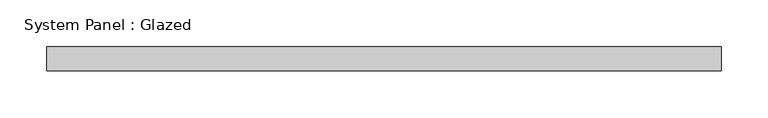
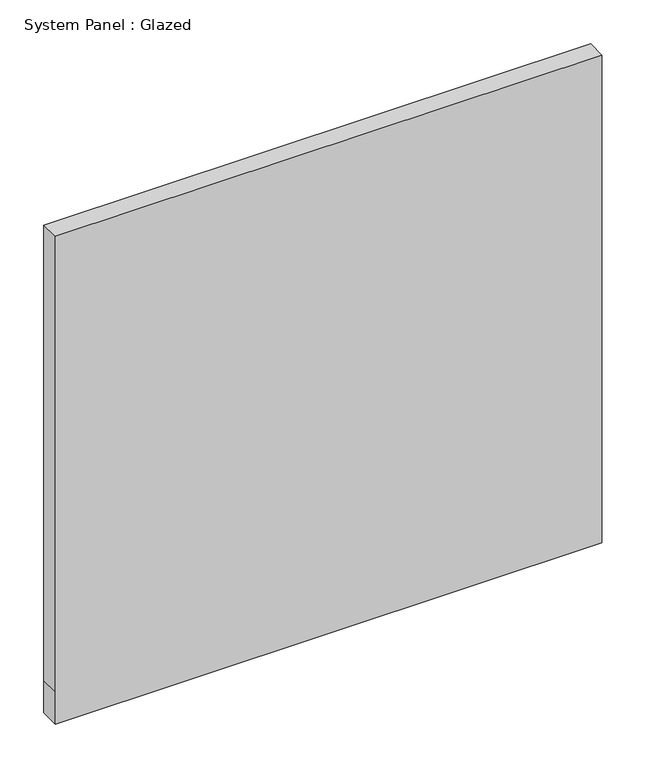
"""IFC4 building model written with IfcOpenShell, lengths in millimetres: plate geometry, System Panel : Glazed."""

from ifc_helpers import new_model, si_unit, frame, origin, place, context, project, spatial, polyline, outline, extrude, source, transform, mapped, element, save


def system_panel_glazed_b40e79ec(model_context):
    return source(origin(), model_context, "Body", "SweptSolid", [
        extrude(outline(polyline([(0.0, -358.775), (0.0, 358.775), (44.45, 358.775), (677.1094531, 358.775), (677.1094531, -358.775), (44.45, -358.775), (0.0, -358.775)])), frame((0.0, 19.05, 0.0), z_axis=(0.0, 1.0, 0.0), x_axis=(0.0, 0.0, 1.0)), (0.0, 0.0, 1.0), 25.4),
    ])


if __name__ == "__main__":
    model = new_model("IFC4")
    model_context = context("Model", 3, world=origin())
    ifc_project = project(units=[si_unit("LENGTHUNIT", "METRE", prefix="MILLI")], contexts=[model_context])
    site = spatial("IfcSite", under=ifc_project)
    building = spatial("IfcBuilding", under=site)
    placement = place(None, origin())
    system_panel_glazed_shape = system_panel_glazed_b40e79ec(model_context)
    element("IfcPlate", 1, ObjectType="System Panel : Glazed", at=placement, inside=building, context=model_context, shape_type="MappedRepresentation", body=[
        mapped(system_panel_glazed_shape, transform((0.0, 0.0, 0.0), x_axis=(1.0, 0.0, 0.0), y_axis=(0.0, 1.0, 0.0), z_axis=(0.0, 0.0, 1.0))),
    ])
    save(model, "model.ifc")

# Revit data of these elements
# Type "System Panel : Glazed"
#   Construction Type Id = "GSP4R"
#   Analytic Construction = "1/8 in Pilkington single glazing"
#   Visual Light Transmittance = 0.9
#   Solar Heat Gain Coefficient = 0.86
#   Heat Transfer Coefficient (U) = 1.18115 BTU/(h·ft²·°F)
#   Define Thermal Properties by = 1
# Element 1 (IfcPlate, "System Panel : Glazed")
#   Materials on its faces: "Glass"
# Materials
#   "Glass": class "Glass", colour RGB 0 128 192, transparency 0.75, Description = "Soda Lime Glass", Cost = 0
